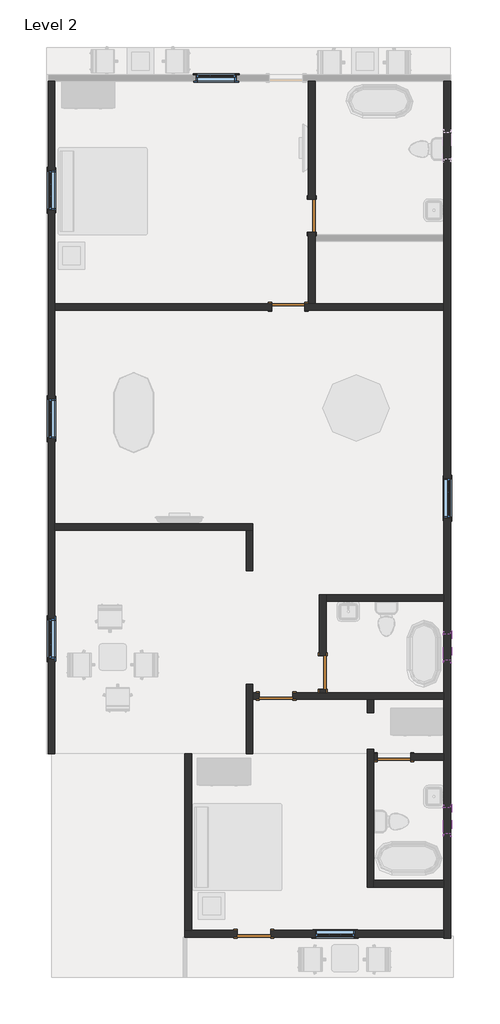
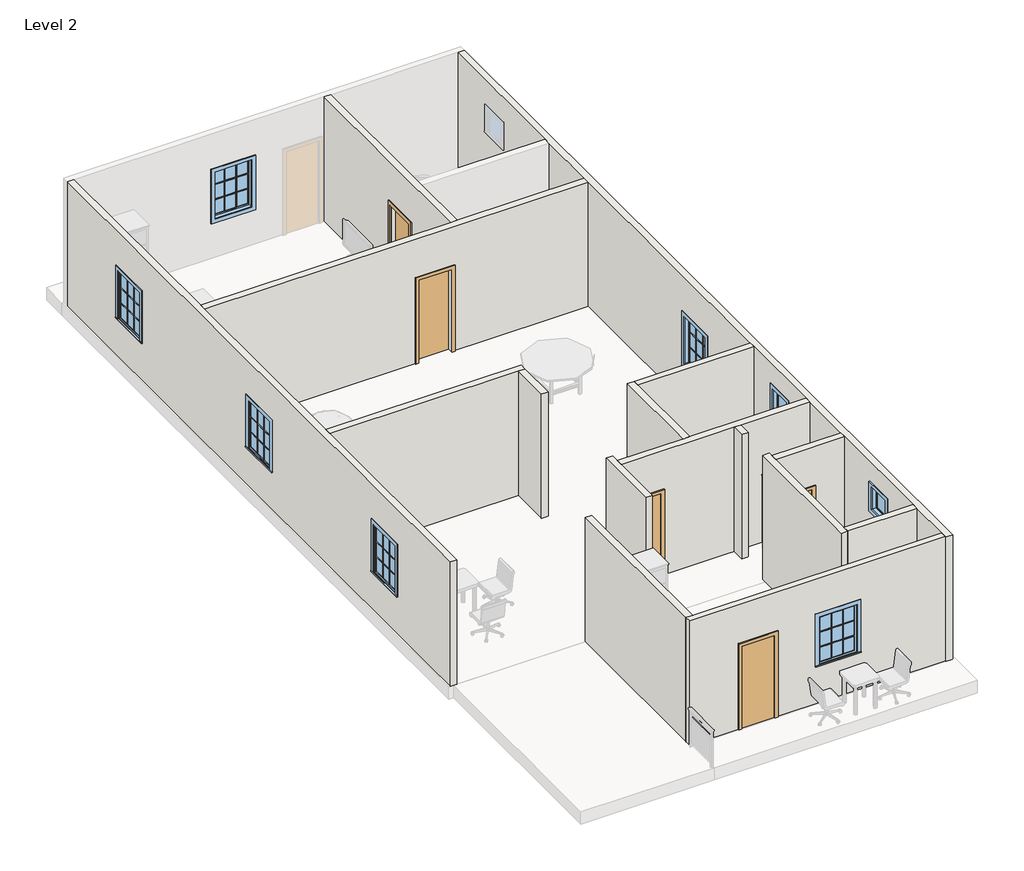
# One storey, part 1 of 2: 16 walls, 8 windows, 6 doors.
"""IFC4 building model written with IfcOpenShell, lengths in millimetres."""

from ifc_helpers import new_model, si_unit, frame, origin, place, context, project, spatial, polyline, outline, extrude, faceted_brep, transform, mapped, element, save
from components import door_059fdd7e, window_5c190c7e, window_3d781103

model = new_model("IFC4")

# Units and contexts
model_context = context("Model", 3, world=origin())
ifc_project = project(units=[si_unit("LENGTHUNIT", "METRE", prefix="MILLI")], contexts=[model_context])

# Site, building, storey
site = spatial("IfcSite", under=ifc_project)
building = spatial("IfcBuilding", under=site)
storey = spatial("IfcBuildingStorey", under=building, Name="Level 2", Elevation=3048.0)

# Doors
placement = place(None, origin())
door_shape = door_059fdd7e(model_context)
element("IfcDoor", 1, ObjectType="Single-Flush : 30\" x 80\"", at=placement, inside=storey, context=model_context, shape_type="MappedRepresentation", body=[
    mapped(door_shape, transform((-7065.3873398, 7157.1549175, 3048.0), x_axis=(1.0, 0.0, 0.0), y_axis=(0.0, 1.0, 0.0), z_axis=(0.0, 0.0, 1.0))),
])
element("IfcDoor", 2, ObjectType="Single-Flush : 30\" x 80\"", at=placement, inside=storey, context=model_context, shape_type="MappedRepresentation", body=[
    mapped(door_shape, transform((-7852.7873398, -7168.4450825, 3048.0), x_axis=(-1.0, 0.0, 0.0), y_axis=(0.0, -1.0, 0.0), z_axis=(0.0, 0.0, 1.0))),
])
element("IfcDoor", 3, ObjectType="Single-Flush : 30\" x 80\"", at=placement, inside=storey, context=model_context, shape_type="MappedRepresentation", body=[
    mapped(door_shape, transform((-4652.3873398, -3129.8450825, 3048.0), x_axis=(-1.0, 0.0, 0.0), y_axis=(0.0, -1.0, 0.0), z_axis=(0.0, 0.0, 1.0))),
])
element("IfcDoor", 4, ObjectType="Single-Flush : 30\" x 80\"", at=placement, inside=storey, context=model_context, shape_type="MappedRepresentation", body=[
    mapped(door_shape, transform((-7344.7873398, -1732.8450825, 3048.0), x_axis=(-1.0, 0.0, 0.0), y_axis=(0.0, -1.0, 0.0), z_axis=(0.0, 0.0, 1.0))),
])
element("IfcDoor", 5, ObjectType="Single-Flush : 30\" x 80\"", at=placement, inside=storey, context=model_context, shape_type="MappedRepresentation", body=[
    mapped(door_shape, transform((-6277.9873398, -1199.4450825, 3048.0), x_axis=(0.0, -1.0, 0.0), y_axis=(1.0, 0.0, 0.0), z_axis=(0.0, 0.0, 1.0))),
])
element("IfcDoor", 6, ObjectType="Single-Flush : 30\" x 80\"", at=placement, inside=storey, context=model_context, shape_type="MappedRepresentation", body=[
    mapped(door_shape, transform((-6531.9873398, 9239.9549175, 3048.0), x_axis=(0.0, -1.0, 0.0), y_axis=(1.0, 0.0, 0.0), z_axis=(0.0, 0.0, 1.0))),
])

# Walls
element("IfcWall", 7, ObjectType="Generic - 8\"", at=placement, inside=storey, context=model_context, shape_type="Brep", body=[
    faceted_brep([(-3509.3873398, 12313.3549175, 3048.0), (-3509.3873398, 8808.1549175, 3048.0), (-3509.3873398, 8655.7549175, 3048.0), (-3509.3873398, 7233.3549175, 3048.0), (-3509.3873398, 7080.9549175, 3048.0), (-3509.3873398, 578.5549175, 3048.0), (-3509.3873398, 426.1549175, 3048.0), (-3509.3873398, -1656.6450825, 3048.0), (-3509.3873398, -1809.0450825, 3048.0), (-3509.3873398, -3053.6450825, 3048.0), (-3509.3873398, -3206.0450825, 3048.0), (-3509.3873398, -5949.2450825, 3048.0), (-3509.3873398, -6101.6450825, 3048.0), (-3509.3873398, -7092.2450825, 3048.0), (-3509.3873398, -7244.6450825, 3048.0), (-3509.3873398, -7270.0450825, 3048.0), (-3509.3873398, -7270.0450825, 6096.0), (-3509.3873398, -7244.6450825, 6096.0), (-3509.3873398, -7092.2450825, 6096.0), (-3509.3873398, -6101.6450825, 6096.0), (-3509.3873398, -5949.2450825, 6096.0), (-3509.3873398, -3206.0450825, 6096.0), (-3509.3873398, -3053.6450825, 6096.0), (-3509.3873398, -1809.0450825, 6096.0), (-3509.3873398, -1656.6450825, 6096.0), (-3509.3873398, 426.1549175, 6096.0), (-3509.3873398, 578.5549175, 6096.0), (-3509.3873398, 7080.9549175, 6096.0), (-3509.3873398, 7233.3549175, 6096.0), (-3509.3873398, 8655.7549175, 6096.0), (-3509.3873398, 8808.1549175, 6096.0), (-3509.3873398, 12313.3549175, 6096.0), (-3509.3873398, 2331.1549175, 5181.6), (-3509.3873398, 2331.1549175, 3962.4), (-3509.3873398, 3245.5549175, 3962.4), (-3509.3873398, 3245.5549175, 5181.6), (-3509.3873398, -4882.4450825, 5562.6), (-3509.3873398, -4882.4450825, 4953.0), (-3509.3873398, -4272.8450825, 4953.0), (-3509.3873398, -4272.8450825, 5562.6), (-3509.3873398, -920.0450825, 5562.6), (-3509.3873398, -920.0450825, 4953.0), (-3509.3873398, -310.4450825, 4953.0), (-3509.3873398, -310.4450825, 5562.6), (-3509.3873398, 11144.9549175, 5435.6), (-3509.3873398, 10535.3549175, 5435.6), (-3509.3873398, 10535.3549175, 4826.0), (-3509.3873398, 11144.9549175, 4826.0), (-3356.9873398, 12313.3549175, 3048.0), (-3356.9873398, 12313.3549175, 6096.0), (-3356.9873398, -7270.0450825, 6096.0), (-3356.9873398, -7270.0450825, 3048.0), (-3356.9873398, 2331.1549175, 5181.6), (-3356.9873398, 3245.5549175, 5181.6), (-3356.9873398, 3245.5549175, 3962.4), (-3356.9873398, 2331.1549175, 3962.4), (-3356.9873398, -4882.4450825, 5562.6), (-3356.9873398, -4272.8450825, 5562.6), (-3356.9873398, -4272.8450825, 4953.0), (-3356.9873398, -4882.4450825, 4953.0), (-3356.9873398, -920.0450825, 5562.6), (-3356.9873398, -310.4450825, 5562.6), (-3356.9873398, -310.4450825, 4953.0), (-3356.9873398, -920.0450825, 4953.0), (-3356.9873398, 11144.9549175, 5435.6), (-3356.9873398, 11144.9549175, 4826.0), (-3356.9873398, 10535.3549175, 4826.0), (-3356.9873398, 10535.3549175, 5435.6)], [[[0, 1, 2, 3, 4, 5, 6, 7, 8, 9, 10, 11, 12, 13, 14, 15, 16, 17, 18, 19, 20, 21, 22, 23, 24, 25, 26, 27, 28, 29, 30, 31], [32, 33, 34, 35], [36, 37, 38, 39], [40, 41, 42, 43], [44, 45, 46, 47]], [[48, 49, 50, 51], [52, 53, 54, 55], [56, 57, 58, 59], [60, 61, 62, 63], [64, 65, 66, 67]], [[15, 14, 13, 12, 11, 10, 9, 8, 7, 6, 5, 4, 3, 2, 1, 0, 48, 51]], [[16, 15, 51, 50]], [[31, 30, 29, 28, 27, 26, 25, 24, 23, 22, 21, 20, 19, 18, 17, 16, 50, 49]], [[0, 31, 49, 48]], [[33, 32, 52, 55]], [[34, 33, 55, 54]], [[35, 34, 54, 53]], [[32, 35, 53, 52]], [[37, 36, 56, 59]], [[38, 37, 59, 58]], [[39, 38, 58, 57]], [[36, 39, 57, 56]], [[41, 40, 60, 63]], [[42, 41, 63, 62]], [[43, 42, 62, 61]], [[40, 43, 61, 60]], [[65, 64, 44, 47]], [[66, 65, 47, 46]], [[67, 66, 46, 45]], [[64, 67, 45, 44]]]),
])
element("IfcWall", 8, ObjectType="Generic - 8\"", at=placement, inside=storey, context=model_context, shape_type="Brep", body=[
    faceted_brep([(-8233.7873398, -7092.2450825, 5080.0), (-8233.7873398, -7092.2450825, 3048.0), (-9275.1873398, -7092.2450825, 3048.0), (-9427.5873398, -7092.2450825, 3048.0), (-9427.5873398, -7092.2450825, 6096.0), (-9275.1873398, -7092.2450825, 6096.0), (-3509.3873398, -7092.2450825, 6096.0), (-3509.3873398, -7092.2450825, 3048.0), (-7471.7873398, -7092.2450825, 3048.0), (-7471.7873398, -7092.2450825, 5080.0), (-6455.7873398, -7092.2450825, 5181.6), (-6455.7873398, -7092.2450825, 3962.4), (-5541.3873398, -7092.2450825, 3962.4), (-5541.3873398, -7092.2450825, 5181.6), (-9427.5873398, -7244.6450825, 3048.0), (-8233.7873398, -7244.6450825, 3048.0), (-8233.7873398, -7244.6450825, 5080.0), (-7471.7873398, -7244.6450825, 5080.0), (-7471.7873398, -7244.6450825, 3048.0), (-3509.3873398, -7244.6450825, 3048.0), (-3509.3873398, -7244.6450825, 6096.0), (-9427.5873398, -7244.6450825, 6096.0), (-6455.7873398, -7244.6450825, 5181.6), (-5541.3873398, -7244.6450825, 5181.6), (-5541.3873398, -7244.6450825, 3962.4), (-6455.7873398, -7244.6450825, 3962.4)], [[[0, 1, 2, 3, 4, 5, 6, 7, 8, 9], [10, 11, 12, 13]], [[14, 15, 16, 17, 18, 19, 20, 21], [22, 23, 24, 25]], [[8, 7, 19, 18]], [[3, 2, 1, 15, 14]], [[6, 5, 4, 21, 20]], [[7, 6, 20, 19]], [[4, 3, 14, 21]], [[16, 15, 1, 0]], [[17, 16, 0, 9]], [[18, 17, 9, 8]], [[11, 10, 22, 25]], [[12, 11, 25, 24]], [[13, 12, 24, 23]], [[10, 13, 23, 22]]]),
])
element("IfcWall", 9, ObjectType="Generic - 8\"", at=placement, inside=storey, context=model_context, shape_type="SweptSolid", body=[
    extrude(outline(polyline([(-9275.1873398, -3053.6450825), (-9275.1873398, -7092.2450825), (-9427.5873398, -7092.2450825), (-9427.5873398, -3053.6450825), (-9275.1873398, -3053.6450825)])), frame((0.0, 0.0, 3048.0), z_axis=(0.0, 0.0, 1.0), x_axis=(1.0, 0.0, 0.0)), (0.0, 0.0, 1.0), 3048.0),
])
element("IfcWall", 10, ObjectType="Generic - 8\"", at=placement, inside=storey, context=model_context, shape_type="Brep", body=[
    faceted_brep([(-6684.3873398, 7080.9549175, 5080.0), (-6684.3873398, 7080.9549175, 3048.0), (-3509.3873398, 7080.9549175, 3048.0), (-3509.3873398, 7080.9549175, 6096.0), (-12399.3873398, 7080.9549175, 6096.0), (-12399.3873398, 7080.9549175, 3048.0), (-7446.3873398, 7080.9549175, 3048.0), (-7446.3873398, 7080.9549175, 5080.0), (-3509.3873398, 7233.3549175, 3048.0), (-6455.7873398, 7233.3549175, 3048.0), (-6608.1873398, 7233.3549175, 3048.0), (-6684.3873398, 7233.3549175, 3048.0), (-6684.3873398, 7233.3549175, 5080.0), (-7446.3873398, 7233.3549175, 5080.0), (-7446.3873398, 7233.3549175, 3048.0), (-12399.3873398, 7233.3549175, 3048.0), (-12399.3873398, 7233.3549175, 6096.0), (-6608.1873398, 7233.3549175, 6096.0), (-6455.7873398, 7233.3549175, 6096.0), (-3509.3873398, 7233.3549175, 6096.0)], [[[0, 1, 2, 3, 4, 5, 6, 7]], [[8, 9, 10, 11, 12, 13, 14, 15, 16, 17, 18, 19]], [[3, 2, 8, 19]], [[12, 11, 1, 0]], [[13, 12, 0, 7]], [[14, 13, 7, 6]], [[6, 5, 15, 14]], [[2, 1, 11, 10, 9, 8]], [[4, 3, 19, 18, 17, 16]], [[5, 4, 16, 15]]]),
])
element("IfcWall", 11, ObjectType="Generic - 8\"", at=placement, inside=storey, context=model_context, shape_type="Brep", body=[
    faceted_brep([(-12399.3873398, 2051.7549175, 3048.0), (-8030.5873398, 2051.7549175, 3048.0), (-7878.1873398, 2051.7549175, 3048.0), (-7878.1873398, 2051.7549175, 6096.0), (-8030.5873398, 2051.7549175, 6096.0), (-12399.3873398, 2051.7549175, 6096.0), (-12399.3873398, 2204.1549175, 3048.0), (-12399.3873398, 2204.1549175, 6096.0), (-7878.1873398, 2204.1549175, 6096.0), (-7878.1873398, 2204.1549175, 3048.0)], [[[0, 1, 2, 3, 4, 5]], [[6, 7, 8, 9]], [[2, 1, 0, 6, 9]], [[5, 4, 3, 8, 7]], [[3, 2, 9, 8]], [[0, 5, 7, 6]]]),
])
element("IfcWall", 12, ObjectType="Generic - 8\"", at=placement, inside=storey, context=model_context, shape_type="SweptSolid", body=[
    extrude(outline(polyline([(-8030.5873398, 1124.6549175), (-8030.5873398, 2051.7549175), (-7878.1873398, 2051.7549175), (-7878.1873398, 1124.6549175), (-8030.5873398, 1124.6549175)])), frame((0.0, 0.0, 3048.0), z_axis=(0.0, 0.0, 1.0), x_axis=(1.0, 0.0, 0.0)), (0.0, 0.0, 1.0), 3048.0),
])
element("IfcWall", 13, ObjectType="Generic - 8\"", at=placement, inside=storey, context=model_context, shape_type="Brep", body=[
    faceted_brep([(-7878.1873398, -1809.0450825, 3048.0), (-7725.7873398, -1809.0450825, 3048.0), (-7725.7873398, -1809.0450825, 5080.0), (-6963.7873398, -1809.0450825, 5080.0), (-6963.7873398, -1809.0450825, 3048.0), (-5261.9873398, -1809.0450825, 3048.0), (-5109.5873398, -1809.0450825, 3048.0), (-3509.3873398, -1809.0450825, 3048.0), (-3509.3873398, -1809.0450825, 6096.0), (-5109.5873398, -1809.0450825, 6096.0), (-5261.9873398, -1809.0450825, 6096.0), (-7878.1873398, -1809.0450825, 6096.0), (-7725.7873398, -1656.6450825, 5080.0), (-7725.7873398, -1656.6450825, 3048.0), (-7878.1873398, -1656.6450825, 3048.0), (-7878.1873398, -1656.6450825, 6096.0), (-6354.1873398, -1656.6450825, 6096.0), (-6201.7873398, -1656.6450825, 6096.0), (-3509.3873398, -1656.6450825, 6096.0), (-3509.3873398, -1656.6450825, 3048.0), (-6201.7873398, -1656.6450825, 3048.0), (-6354.1873398, -1656.6450825, 3048.0), (-6963.7873398, -1656.6450825, 3048.0), (-6963.7873398, -1656.6450825, 5080.0)], [[[0, 1, 2, 3, 4, 5, 6, 7, 8, 9, 10, 11]], [[12, 13, 14, 15, 16, 17, 18, 19, 20, 21, 22, 23]], [[14, 13, 1, 0]], [[22, 21, 20, 19, 7, 6, 5, 4]], [[11, 10, 9, 8, 18, 17, 16, 15]], [[8, 7, 19, 18]], [[0, 11, 15, 14]], [[2, 1, 13, 12]], [[3, 2, 12, 23]], [[4, 3, 23, 22]]]),
])
element("IfcWall", 14, ObjectType="Generic - 8\"", at=placement, inside=storey, context=model_context, shape_type="SweptSolid", body=[
    extrude(outline(polyline([(-5261.9873398, -2113.8450825), (-5261.9873398, -1809.0450825), (-5109.5873398, -1809.0450825), (-5109.5873398, -2113.8450825), (-5261.9873398, -2113.8450825)])), frame((0.0, 0.0, 3048.0), z_axis=(0.0, 0.0, 1.0), x_axis=(1.0, 0.0, 0.0)), (0.0, 0.0, 1.0), 3048.0),
])
element("IfcWall", 15, ObjectType="Generic - 8\"", at=placement, inside=storey, context=model_context, shape_type="SweptSolid", body=[
    extrude(outline(polyline([(-3509.3873398, -6101.6450825), (-5109.5873398, -6101.6450825), (-5109.5873398, -5949.2450825), (-3509.3873398, -5949.2450825), (-3509.3873398, -6101.6450825)])), frame((0.0, 0.0, 3048.0), z_axis=(0.0, 0.0, 1.0), x_axis=(1.0, 0.0, 0.0)), (0.0, 0.0, 1.0), 3048.0),
])
element("IfcWall", 16, ObjectType="Generic - 8\"", at=placement, inside=storey, context=model_context, shape_type="SweptSolid", body=[
    extrude(outline(polyline([(3048.0, -5109.5873398), (3048.0, -5033.3873398), (5080.0, -5033.3873398), (5080.0, -4271.3873398), (3048.0, -4271.3873398), (3048.0, -3509.3873398), (6096.0, -3509.3873398), (6096.0, -5109.5873398), (3048.0, -5109.5873398)])), frame((0.0, -3206.0450825, 0.0), z_axis=(0.0, 1.0, 0.0), x_axis=(0.0, 0.0, 1.0)), (0.0, 0.0, 1.0), 152.4),
])
element("IfcWall", 17, ObjectType="Generic - 8\"", at=placement, inside=storey, context=model_context, shape_type="Brep", body=[
    faceted_brep([(-6201.7873398, -1656.6450825, 3048.0), (-6201.7873398, -1580.4450825, 3048.0), (-6201.7873398, -1580.4450825, 5080.0), (-6201.7873398, -818.4450825, 5080.0), (-6201.7873398, -818.4450825, 3048.0), (-6201.7873398, 426.1549175, 3048.0), (-6201.7873398, 578.5549175, 3048.0), (-6201.7873398, 578.5549175, 6096.0), (-6201.7873398, 426.1549175, 6096.0), (-6201.7873398, -1656.6450825, 6096.0), (-6354.1873398, -1580.4450825, 5080.0), (-6354.1873398, -1580.4450825, 3048.0), (-6354.1873398, -1656.6450825, 3048.0), (-6354.1873398, -1656.6450825, 6096.0), (-6354.1873398, 578.5549175, 6096.0), (-6354.1873398, 578.5549175, 3048.0), (-6354.1873398, -818.4450825, 3048.0), (-6354.1873398, -818.4450825, 5080.0)], [[[0, 1, 2, 3, 4, 5, 6, 7, 8, 9]], [[10, 11, 12, 13, 14, 15, 16, 17]], [[16, 15, 6, 5, 4]], [[12, 11, 1, 0]], [[9, 8, 7, 14, 13]], [[0, 9, 13, 12]], [[7, 6, 15, 14]], [[2, 1, 11, 10]], [[3, 2, 10, 17]], [[4, 3, 17, 16]]]),
])
element("IfcWall", 18, ObjectType="Generic - 8\"", at=placement, inside=storey, context=model_context, shape_type="SweptSolid", body=[
    extrude(outline(polyline([(-3509.3873398, 426.1549175), (-6201.7873398, 426.1549175), (-6201.7873398, 578.5549175), (-3509.3873398, 578.5549175), (-3509.3873398, 426.1549175)])), frame((0.0, 0.0, 3048.0), z_axis=(0.0, 0.0, 1.0), x_axis=(1.0, 0.0, 0.0)), (0.0, 0.0, 1.0), 3048.0),
])
element("IfcWall", 19, ObjectType="Generic - 8\"", at=placement, inside=storey, context=model_context, shape_type="Brep", body=[
    faceted_brep([(-6455.7873398, 7233.3549175, 3048.0), (-6455.7873398, 8655.7549175, 3048.0), (-6455.7873398, 8808.1549175, 3048.0), (-6455.7873398, 8858.9549175, 3048.0), (-6455.7873398, 8858.9549175, 5080.0), (-6455.7873398, 9620.9549175, 5080.0), (-6455.7873398, 9620.9549175, 3048.0), (-6455.7873398, 12313.3549175, 3048.0), (-6455.7873398, 12313.3549175, 6096.0), (-6455.7873398, 8808.1549175, 6096.0), (-6455.7873398, 8655.7549175, 6096.0), (-6455.7873398, 7233.3549175, 6096.0), (-6608.1873398, 8858.9549175, 5080.0), (-6608.1873398, 8858.9549175, 3048.0), (-6608.1873398, 7233.3549175, 3048.0), (-6608.1873398, 7233.3549175, 6096.0), (-6608.1873398, 12313.3549175, 6096.0), (-6608.1873398, 12313.3549175, 3048.0), (-6608.1873398, 9620.9549175, 3048.0), (-6608.1873398, 9620.9549175, 5080.0)], [[[0, 1, 2, 3, 4, 5, 6, 7, 8, 9, 10, 11]], [[12, 13, 14, 15, 16, 17, 18, 19]], [[18, 17, 7, 6]], [[14, 13, 3, 2, 1, 0]], [[11, 10, 9, 8, 16, 15]], [[8, 7, 17, 16]], [[0, 11, 15, 14]], [[4, 3, 13, 12]], [[5, 4, 12, 19]], [[6, 5, 19, 18]]]),
])
element("IfcWall", 20, ObjectType="Generic - 8\"", at=placement, inside=storey, context=model_context, shape_type="Brep", body=[
    faceted_brep([(-5261.9873398, -2952.0450825, 3048.0), (-5261.9873398, -6101.6450825, 3048.0), (-5261.9873398, -6101.6450825, 6096.0), (-5261.9873398, -2952.0450825, 6096.0), (-5109.5873398, -2952.0450825, 3048.0), (-5109.5873398, -2952.0450825, 6096.0), (-5109.5873398, -3053.6450825, 6096.0), (-5109.5873398, -3206.0450825, 6096.0), (-5109.5873398, -5949.2450825, 6096.0), (-5109.5873398, -6101.6450825, 6096.0), (-5109.5873398, -6101.6450825, 3048.0), (-5109.5873398, -5949.2450825, 3048.0), (-5109.5873398, -3206.0450825, 3048.0), (-5109.5873398, -3053.6450825, 3048.0)], [[[0, 1, 2, 3]], [[4, 5, 6, 7, 8, 9, 10, 11, 12, 13]], [[1, 0, 4, 13, 12, 11, 10]], [[3, 2, 9, 8, 7, 6, 5]], [[0, 3, 5, 4]], [[2, 1, 10, 9]]]),
])
element("IfcWall", 21, ObjectType="Generic - 8\"", at=placement, inside=storey, context=model_context, shape_type="Brep", body=[
    faceted_brep([(-8030.5873398, -1466.1450825, 3048.0), (-8030.5873398, -3053.6450825, 3048.0), (-8030.5873398, -3053.6450825, 6096.0), (-8030.5873398, -1466.1450825, 6096.0), (-7878.1873398, -1466.1450825, 3048.0), (-7878.1873398, -1466.1450825, 6096.0), (-7878.1873398, -1656.6450825, 6096.0), (-7878.1873398, -1809.0450825, 6096.0), (-7878.1873398, -3053.6450825, 6096.0), (-7878.1873398, -3053.6450825, 3048.0), (-7878.1873398, -1809.0450825, 3048.0), (-7878.1873398, -1656.6450825, 3048.0)], [[[0, 1, 2, 3]], [[4, 5, 6, 7, 8, 9, 10, 11]], [[1, 0, 4, 11, 10, 9]], [[2, 1, 9, 8]], [[3, 2, 8, 7, 6, 5]], [[0, 3, 5, 4]]]),
])
element("IfcWall", 22, ObjectType="Generic - 8\"", at=placement, inside=storey, context=model_context, shape_type="Brep", body=[
    faceted_brep([(-12551.7873398, 12313.3549175, 3048.0), (-12551.7873398, -3053.6450825, 3048.0), (-12551.7873398, -3053.6450825, 6096.0), (-12551.7873398, 12313.3549175, 6096.0), (-12551.7873398, 10281.3549175, 5181.6), (-12551.7873398, 9366.9549175, 5181.6), (-12551.7873398, 9366.9549175, 3962.4), (-12551.7873398, 10281.3549175, 3962.4), (-12551.7873398, 32.4549175, 5181.6), (-12551.7873398, -881.9450825, 5181.6), (-12551.7873398, -881.9450825, 3962.4), (-12551.7873398, 32.4549175, 3962.4), (-12551.7873398, 5061.6549175, 5181.6), (-12551.7873398, 4147.2549175, 5181.6), (-12551.7873398, 4147.2549175, 3962.4), (-12551.7873398, 5061.6549175, 3962.4), (-12399.3873398, 12313.3549175, 3048.0), (-12399.3873398, 12313.3549175, 6096.0), (-12399.3873398, 7233.3549175, 6096.0), (-12399.3873398, 7080.9549175, 6096.0), (-12399.3873398, 2204.1549175, 6096.0), (-12399.3873398, 2051.7549175, 6096.0), (-12399.3873398, -3053.6450825, 6096.0), (-12399.3873398, -3053.6450825, 3048.0), (-12399.3873398, 2051.7549175, 3048.0), (-12399.3873398, 2204.1549175, 3048.0), (-12399.3873398, 7080.9549175, 3048.0), (-12399.3873398, 7233.3549175, 3048.0), (-12399.3873398, 10281.3549175, 5181.6), (-12399.3873398, 10281.3549175, 3962.4), (-12399.3873398, 9366.9549175, 3962.4), (-12399.3873398, 9366.9549175, 5181.6), (-12399.3873398, 32.4549175, 5181.6), (-12399.3873398, 32.4549175, 3962.4), (-12399.3873398, -881.9450825, 3962.4), (-12399.3873398, -881.9450825, 5181.6), (-12399.3873398, 5061.6549175, 5181.6), (-12399.3873398, 5061.6549175, 3962.4), (-12399.3873398, 4147.2549175, 3962.4), (-12399.3873398, 4147.2549175, 5181.6)], [[[0, 1, 2, 3], [4, 5, 6, 7], [8, 9, 10, 11], [12, 13, 14, 15]], [[16, 17, 18, 19, 20, 21, 22, 23, 24, 25, 26, 27], [28, 29, 30, 31], [32, 33, 34, 35], [36, 37, 38, 39]], [[1, 0, 16, 27, 26, 25, 24, 23]], [[2, 1, 23, 22]], [[3, 2, 22, 21, 20, 19, 18, 17]], [[0, 3, 17, 16]], [[29, 28, 4, 7]], [[30, 29, 7, 6]], [[31, 30, 6, 5]], [[28, 31, 5, 4]], [[33, 32, 8, 11]], [[34, 33, 11, 10]], [[35, 34, 10, 9]], [[32, 35, 9, 8]], [[37, 36, 12, 15]], [[38, 37, 15, 14]], [[39, 38, 14, 13]], [[36, 39, 13, 12]]]),
])

# Windows
window_shape = window_5c190c7e(model_context)
element("IfcWindow", 23, ObjectType="Casement 3x3 with Trim : 36\" x 48\"", at=placement, inside=storey, context=model_context, shape_type="MappedRepresentation", body=[
    mapped(window_shape, transform((-8716.3873398, 12389.5549175, 3048.0), x_axis=(1.0, 0.0, 0.0), y_axis=(0.0, 1.0, 0.0), z_axis=(0.0, 0.0, 1.0))),
])
element("IfcWindow", 24, ObjectType="Casement 3x3 with Trim : 36\" x 48\"", at=placement, inside=storey, context=model_context, shape_type="MappedRepresentation", body=[
    mapped(window_shape, transform((-5998.5873398, -7168.4450825, 3048.0), x_axis=(-1.0, 0.0, 0.0), y_axis=(0.0, -1.0, 0.0), z_axis=(0.0, 0.0, 1.0))),
])
element("IfcWindow", 25, ObjectType="Casement 3x3 with Trim : 36\" x 48\"", at=placement, inside=storey, context=model_context, shape_type="MappedRepresentation", body=[
    mapped(window_shape, transform((-3433.1873398, 2788.3549175, 3048.0), x_axis=(0.0, -1.0, 0.0), y_axis=(1.0, 0.0, 0.0), z_axis=(0.0, 0.0, 1.0))),
])
element("IfcWindow", 26, ObjectType="Casement 3x3 with Trim : 36\" x 48\"", at=placement, inside=storey, context=model_context, shape_type="MappedRepresentation", body=[
    mapped(window_shape, transform((-12475.5873398, 4604.4549175, 3048.0), x_axis=(0.0, 1.0, 0.0), y_axis=(-1.0, 0.0, 0.0), z_axis=(0.0, 0.0, 1.0))),
])
element("IfcWindow", 27, ObjectType="Casement 3x3 with Trim : 36\" x 48\"", at=placement, inside=storey, context=model_context, shape_type="MappedRepresentation", body=[
    mapped(window_shape, transform((-12475.5873398, -424.7450825, 3048.0), x_axis=(0.0, 1.0, 0.0), y_axis=(-1.0, 0.0, 0.0), z_axis=(0.0, 0.0, 1.0))),
])
element("IfcWindow", 28, ObjectType="Casement 3x3 with Trim : 36\" x 48\"", at=placement, inside=storey, context=model_context, shape_type="MappedRepresentation", body=[
    mapped(window_shape, transform((-12475.5873398, 9824.1549175, 3048.0), x_axis=(0.0, 1.0, 0.0), y_axis=(-1.0, 0.0, 0.0), z_axis=(0.0, 0.0, 1.0))),
])
window_2_shape = window_3d781103(model_context)
element("IfcWindow", 29, ObjectType="Transom with Trim : 24\" x 24\"", at=placement, inside=storey, context=model_context, shape_type="MappedRepresentation", body=[
    mapped(window_2_shape, transform((-3433.1873398, -4615.7450825, 2794.0), x_axis=(0.0, -1.0, 0.0), y_axis=(1.0, 0.0, 0.0), z_axis=(0.0, 0.0, 1.0))),
])
element("IfcWindow", 30, ObjectType="Transom with Trim : 24\" x 24\"", at=placement, inside=storey, context=model_context, shape_type="MappedRepresentation", body=[
    mapped(window_2_shape, transform((-3433.1873398, -653.3450825, 2794.0), x_axis=(0.0, -1.0, 0.0), y_axis=(1.0, 0.0, 0.0), z_axis=(0.0, 0.0, 1.0))),
])

save(model, "model.ifc")

# Revit data of these elements
# Type "Single-Flush : 30\" x 80\""
#   Type Mark = "5"
#   Construction Type Id = "MDOOR"
#   Assembly Code = "C1020"
#   Analytic Construction = "Metal"
#   Thickness = 0' - 2"
#   Heat Transfer Coefficient (U) = 0.651978 BTU/(h·ft²·°F)
#   Height = 6' - 8"
#   Trim Projection Ext = 0' - 1"
#   Trim Projection Int = 0' - 1"
#   Trim Width = 0' - 3"
#   Width = 2' - 6"
#   Define Thermal Properties by = 1
#   Door Material = Door - Panel
#   Frame Material = Door - Frame
#   Visual Light Transmittance = 0
#   Solar Heat Gain Coefficient = 0
#   Function = (empty or 0)
#   Wall Closure = (empty or 0)
# Type "Generic - 8\""
#   Assembly Code = "B2010"
#   Layers, outside or top first: 0' - 6" "Brick, Common" (function 1)
# Type "Casement 3x3 with Trim : 36\" x 48\""
#   Type Mark = "10"
#   Construction Type Id = "GSP4R"
#   Assembly Code = "B2020100"
#   Analytic Construction = "1/8 in Pilkington single glazing"
#   Visual Light Transmittance = 0.9
#   Solar Heat Gain Coefficient = 0.78
#   Heat Transfer Coefficient (U) = 0.6496 BTU/(h·ft²·°F)
#   Height = 4' - 0"
#   Default Sill Height = 3' - 0"
#   Trim Projection - Ext. = 0' - 0 1/2"
#   Trim Projection - Int. = 0' - 0 3/4"
#   Trim Width - Exterior = 0' - 3 1/2"
#   Trim Width - Interior = 0' - 3 1/2"
#   Width = 3' - 0"
#   Window Inset = 0' - 0 3/4"
#   Define Thermal Properties by = 1
#   Glass Pane Material = Glass
#   Sash Material = Sash
#   Trim Exterior Material = Trim
#   Trim Interior Material = Trim
#   Wall Closure = (empty or 0)
# Type "Transom with Trim : 24\" x 24\""
#   Type Mark = "13"
#   Construction Type Id = "GSP4R"
#   Assembly Code = "B2020100"
#   Analytic Construction = "1/8 in Pilkington single glazing"
#   Visual Light Transmittance = 0.9
#   Solar Heat Gain Coefficient = 0.78
#   Heat Transfer Coefficient (U) = 0.6496 BTU/(h·ft²·°F)
#   Height = 2' - 0"
#   Default Sill Height = 7' - 1"
#   Trim Projection - Ext. = 0' - 0 1/2"
#   Trim Projection - Int. = 0' - 0 3/4"
#   Trim Width - Exterior = 0' - 3 1/2"
#   Trim Width - Interior = 0' - 3 1/2"
#   Width = 2' - 0"
#   Window Inset = 0' - 0 3/4"
#   Define Thermal Properties by = 1
#   Glass Pane Material = Glass
#   Sash Material = Sash
#   Trim Exterior Material = Trim
#   Trim Interior Material = Trim
#   Wall Closure = (empty or 0)
# Elements 1, 2, 3, 4, 5, 6 (IfcDoor, "Single-Flush : 30\" x 80\"")
#   Phase Created = New Construction
#   Materials on its faces: "Door - Frame", "Door - Panel"
# Elements 7, 8, 9, 10, 11, 12, 13, 14, 15, 16, 17, 18, 19, 20, 21, 22 (IfcWall, "Generic - 8\"")
#   Top Offset = 0' - 0"
#   Base Offset = 0' - 0"
#   Unconnected Height = 10' - 0"
#   wall height = 10' - 0"
#   Phase Created = New Construction
#   Base Constraint = Level 2
#   Materials on its faces: "Brick, Common"
# Element 23 (IfcWindow, "Casement 3x3 with Trim : 36\" x 48\"")
#   Mark = "14"
#   Phase Created = New Construction
#   Materials on its faces: "Sash", "Glass", "Trim"
# Element 24 (IfcWindow, "Casement 3x3 with Trim : 36\" x 48\"")
#   Mark = "15"
#   Phase Created = New Construction
#   Materials on its faces: "Sash", "Glass", "Trim"
# Element 25 (IfcWindow, "Casement 3x3 with Trim : 36\" x 48\"")
#   Mark = "16"
#   Phase Created = New Construction
#   Materials on its faces: "Sash", "Glass", "Trim"
# Element 26 (IfcWindow, "Casement 3x3 with Trim : 36\" x 48\"")
#   Mark = "22"
#   Phase Created = New Construction
#   Materials on its faces: "Sash", "Glass", "Trim"
# Element 27 (IfcWindow, "Casement 3x3 with Trim : 36\" x 48\"")
#   Mark = "23"
#   Phase Created = New Construction
#   Materials on its faces: "Sash", "Glass", "Trim"
# Element 28 (IfcWindow, "Casement 3x3 with Trim : 36\" x 48\"")
#   Mark = "24"
#   Phase Created = New Construction
#   Materials on its faces: "Sash", "Glass", "Trim"
# Element 29 (IfcWindow, "Transom with Trim : 24\" x 24\"")
#   Mark = "19"
#   Phase Created = New Construction
#   Materials on its faces: "Sash", "Trim", "Glass"
# Element 30 (IfcWindow, "Transom with Trim : 24\" x 24\"")
#   Mark = "20"
#   Phase Created = New Construction
#   Materials on its faces: "Sash", "Trim", "Glass"
# Materials
#   "Door - Panel": class "Wood", colour RGB 210 159 95, transparency 0
#   "Door - Frame": colour RGB 118 70 51, transparency 0
#   "Brick, Common": class "Masonry", colour RGB 170 98 104, transparency 0, Description = "Common brick", Cost = 0
#   "Glass": class "Glass", colour RGB 0 128 192, transparency 0.75, Description = "Soda Lime Glass", Cost = 0
#   "Sash": class "Wood", colour RGB 224 178 126, transparency 0
#   "Trim": class "Wood", colour RGB 224 178 126, transparency 0
# Room at (-7884.301, 12599.648) mm, phase "New Construction", upper level "Level 2", upper offset 10' - 0", lower offset 0' - 0"
#   Number = "14"
#   Name = "BALCONY"
# Room at (-5133.338, 10089.997) mm, phase "New Construction", upper level "Level 2", upper offset 10' - 0", lower offset 0' - 0"
#   Number = "16"
#   Name = "TOILET"
# Room at (-8994.339, 10089.997) mm, phase "New Construction", upper level "Level 2", upper offset 10' - 0", lower offset 0' - 0"
#   Number = "15"
#   Name = "BEDROOM"
# Room at (-9713.101, 4274.364) mm, phase "New Construction", upper level "Level 2", upper offset 10' - 0", lower offset 0' - 0"
#   Number = "18"
#   Name = "LIVING"
# Room at (-6962.138, 4274.364) mm, phase "New Construction", upper level "Level 2", upper offset 10' - 0", lower offset 0' - 0"
#   Number = "19"
#   Name = "DINING"
# Room at (-4723.106, -769.068) mm, phase "New Construction", upper level "Level 2", upper offset 10' - 0", lower offset 0' - 0"
#   Number = "20"
# Room at (-10200.902, -431.231) mm, phase "New Construction", upper level "Level 2", upper offset 10' - 0", lower offset 0' - 0"
#   Number = "21"
#   Name = "TERRACE SITE"
# Room at (-10973.102, -5209.22) mm, phase "New Construction", upper level "Level 2", upper offset 10' - 0", lower offset 0' - 0"
#   Number = "22"
#   Name = "OPEN TERRACE GARDEN"
# Room at (-6962.138, -4581.807) mm, phase "New Construction", upper level "Level 2", upper offset 10' - 0", lower offset 0' - 0"
#   Number = "23"
#   Name = "BEDROOM"
# Room at (-4312.875, -4581.807) mm, phase "New Construction", upper level "Level 2", upper offset 10' - 0", lower offset 0' - 0"
#   Number = "24"
# Room at (-5591.832, -7839.527) mm, phase "New Construction", upper level "Level 2", upper offset 10' - 0", lower offset 0' - 0"
#   Number = "25"
#   Name = "BALCONY"
# Room at (-4312.875, -2361.731) mm, phase "New Construction", upper level "Level 2", upper offset 10' - 0", lower offset 0' - 0"
#   Number = "26"
# Room at (-5133.338, 7918.184) mm, phase "New Construction", upper level "Level 2", upper offset 10' - 0", lower offset 0' - 0"
#   Number = "17"
#   Name = "DUCT"
